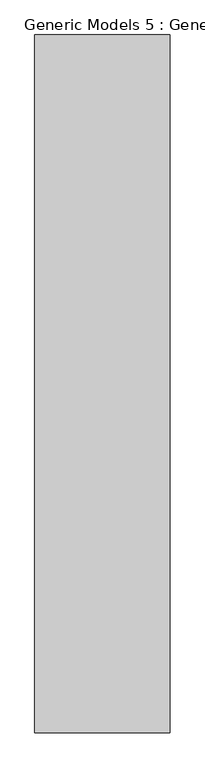
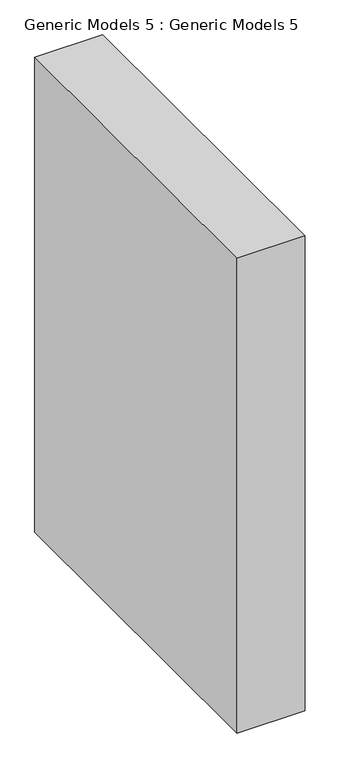
"""IFC4 building model written with IfcOpenShell, lengths in millimetres: proxy geometry, Generic Models 5 : Generic Models 5."""

from ifc_helpers import new_model, si_unit, origin, place, context, project, spatial, faceted_brep, source, transform, mapped, element, save


def generic_models_5_generic_models_5_b383e08d(model_context):
    return source(origin(), model_context, "Body", "Brep", [
        faceted_brep([(-16587.1168969, -15333.7742702, 9460.6359555), (-16587.1168969, -13196.1337862, 9460.6359555), (-17001.1767684, -13196.1337862, 9460.6359555), (-17001.1767684, -15333.7742702, 9460.6359555), (-16587.1168969, -15333.7742702, 6400.8), (-17001.1767684, -15333.7742702, 6400.8), (-17001.1767684, -13196.1337862, 6400.8), (-16587.1168969, -13196.1337862, 6400.8), (-16587.1168969, -13196.1337862, 9451.4798658), (-17001.1767684, -13196.1337862, 9451.4798658)], [[[0, 1, 2, 3]], [[4, 5, 6, 7]], [[1, 0, 4, 7, 8]], [[2, 1, 8, 7, 6, 9]], [[3, 2, 9, 6, 5]], [[0, 3, 5, 4]]]),
    ])


if __name__ == "__main__":
    model = new_model("IFC4")
    model_context = context("Model", 3, world=origin())
    ifc_project = project(units=[si_unit("LENGTHUNIT", "METRE", prefix="MILLI")], contexts=[model_context])
    site = spatial("IfcSite", under=ifc_project)
    building = spatial("IfcBuilding", under=site)
    placement = place(None, origin())
    generic_models_5_generic_models_5_shape = generic_models_5_generic_models_5_b383e08d(model_context)
    element("IfcBuildingElementProxy", 1, Name="Generic Models 5 : Generic Models 5", ObjectType="Generic Models 5 : Generic Models 5", at=placement, inside=building, context=model_context, shape_type="MappedRepresentation", body=[
        mapped(generic_models_5_generic_models_5_shape, transform((0.0, 0.0, 0.0), x_axis=(1.0, 0.0, 0.0), y_axis=(0.0, 1.0, 0.0), z_axis=(0.0, 0.0, 1.0))),
    ])
    save(model, "model.ifc")
